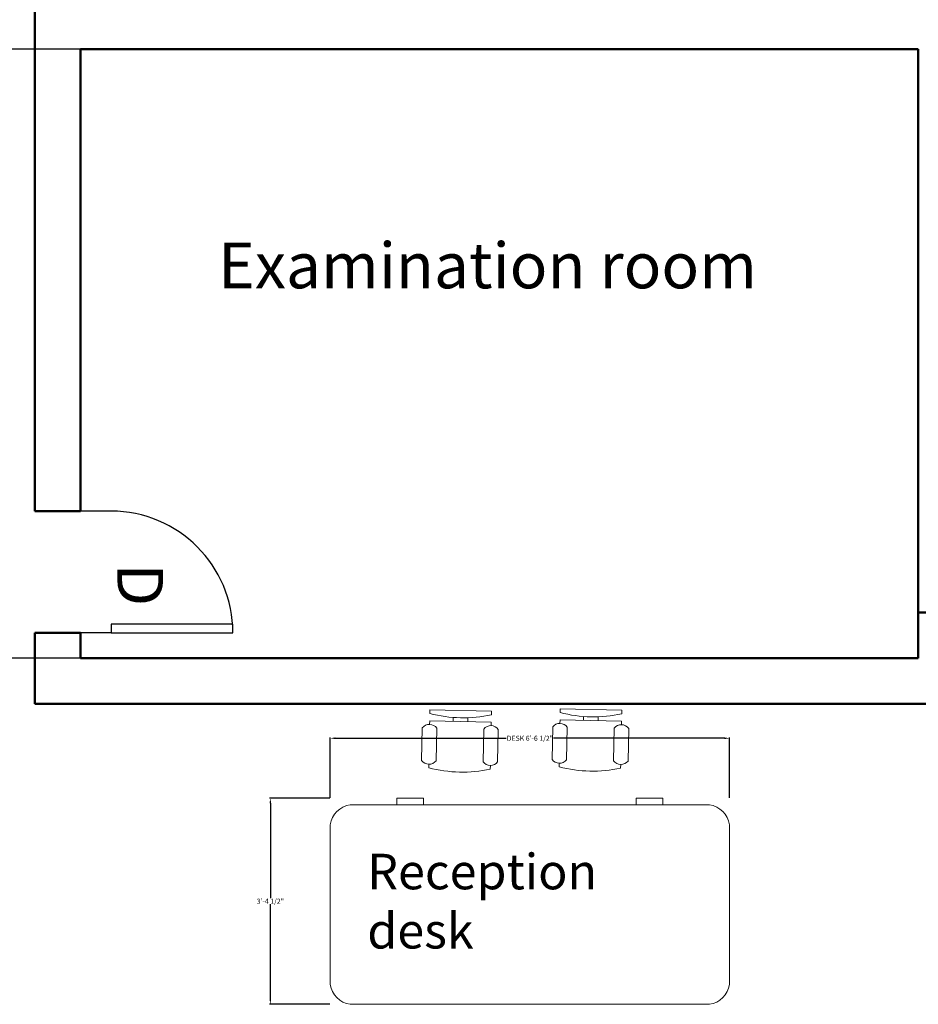
# Model space of a CAD drawing. Units: inches. Extents: x -364 to 705, y -52 to 1250.
# Tile 15 of 34: x 182 to 359, y 454 to 648. Entities that reach past the tile are written whole.
import ezdxf

# ---------------------------------------------------------------- set-up
doc = ezdxf.new("R2010")
doc.units = ezdxf.units.IN
doc.header["$MEASUREMENT"] = 0
for name, color, linetype, lineweight in [('A-ANNO-DIMS', 4, 'Continuous', 18), ('A-ANNO-IDEN', 1, 'Continuous', 18), ('A-ANNO-TEXT', 3, 'Continuous', 18), ('A-AREA-IDEN', 3, 'Continuous', 18), ('A-DOOR', 1, 'Continuous', 25), ('A-FURN', 8, 'Continuous', 18), ('A-WALL', 41, 'Continuous', 50)]:
    doc.layers.add(name, color=color, linetype=linetype, lineweight=lineweight)
doc.styles.get("Standard").update_dxf_attribs({"font": 'arial.ttf'})
doc.dimstyles.get("Standard").update_dxf_attribs({"dimtxt": 1, "dimasz": 1, "dimexe": 0.18, "dimexo": 0.0625, "dimgap": 0.09, "dimtad": 0, "dimtih": 1, "dimtoh": 1, "dimdec": 0, "dimzin": 0, "dimdsep": 46, "dimlunit": 3, "dimtxsty": 'Standard', "dimcen": 0.09, "dimadec": 0, "dimazin": 0, "dimtfac": 1, "dimtdec": 0, "dimtofl": 0, "dimtmove": 0, "dimatfit": 3, "dimfxl": 1, "dimtolj": 1, "dimtzin": 0, "dimarcsym": 0})

# ---------------------------------------------------------------- blocks, each defined once
blk = doc.blocks.new('*U14')
for p, q in [((0, 0), (0, -6)), ((-24, 0), (-24, -6))]:
    blk.add_line(p, q)
blk.add_lwpolyline([(0, 0), (0, 24), (-1.75, 24), (-1.75, 0)], close=True)
blk.add_arc((0, 0), 24, 90, 180)
blk = doc.blocks.new('Chair - Desk')
for p, q in [((-8.5, 0), (-8.5, -1)), ((-8.5, 0), (8.5, 0)), ((8.5, 0), (8.5, -1)), ((-2, -3), (-2, -1.9355)), ((2, -1.9576), (2, -3)), ((-10.5, -5), (-10.5, -14)), ((-8.5, -3), (-8.5, -4)), ((-8.5, -3), (8.5, -3)), ((-6.5, -14), (-6.5, -5)), ((6.5, -5), (6.5, -14)), ((8.5, -3), (8.5, -4)), ((10.5, -14), (10.5, -5)), ((-8.5, -15), (-8.5, -16)), ((8.5, -15), (8.5, -16))]:
    blk.add_line(p, q)
for centre, radius, start, end in [((0, 34.625), 36.625, 256.5803, 283.4197), ((-8.5, -6.5), 2.5, 36.8699, 143.1301), ((8.5, -6.5), 2.5, 36.8699, 143.1301), ((-8.5, -12.5), 2.5, 216.8699, 323.1301), ((0, 19.625), 36.625, 256.5803, 283.4197), ((8.5, -12.5), 2.5, 216.8699, 323.1301)]:
    blk.add_arc(centre, radius, start, end)
blk = doc.blocks.new('Desk - 30 x 60 in.')
for p, q in [((-26.999995, 0), (26.999995, 0)), ((-29.999995, -27), (-29.999995, -3)), ((29.999995, -3), (29.999995, -27)), ((26.999995, -30), (-26.999995, -30)), ((-20.000005, -30), (-20.000005, -31)), ((-20.000005, -31), (-16.000005, -31)), ((-16.000005, -31), (-16.000005, -30)), ((15.999995, -31), (15.999995, -30)), ((19.999995, -31), (15.999995, -31)), ((19.999995, -30), (19.999995, -31))]:
    blk.add_line(p, q)
for centre, start, end in [((-26.499995, -3.5), 98.1301, 171.8699), ((26.499995, -3.5), 8.130102, 81.8699), ((-26.499995, -26.5), 188.1301, 261.8699), ((26.499995, -26.5), 278.1301, 351.8699)]:
    blk.add_arc(centre, 3.535534, start, end)
blk = doc.blocks.new('*D50')
at = {"layer": 'A-ANNO-DIMS', "color": 0, "lineweight": -2, "transparency": 16777216}
for p, q in [((242.75, 494.62), (242.75, 506.53)), ((321.38, 494.62), (321.38, 506.53)), ((243.75, 506.35), (277.41, 506.35)), ((320.38, 506.35), (286.72, 506.35))]:
    blk.add_line(p, q, dxfattribs=at)
at = {"layer": 'A-ANNO-DIMS', "color": 0, "transparency": 16777216}
for points in [[(243.75, 506.52), (243.75, 506.19), (242.75, 506.35)], [(320.38, 506.52), (320.38, 506.19), (321.38, 506.35)]]:
    blk.add_solid(points, dxfattribs=at)
at = {"layer": 'Defpoints', "color": 0, "transparency": 16777216}
for p in [(242.75, 506.35), (242.75, 494.56), (321.38, 494.56)]:
    blk.add_point(p, dxfattribs=at)
at = {"layer": 'A-ANNO-DIMS', "color": 0, "transparency": 16777216, "insert": (282.07, 506.35), "char_height": 1, "attachment_point": 5}
blk.add_mtext('\\A1;DESK 6\'-6 1/2"', dxfattribs=at)
blk = doc.blocks.new('*D51')
at = {"layer": 'A-ANNO-DIMS', "color": 0, "lineweight": -2, "transparency": 16777216}
for p, q in [((242.69, 494.56), (230.77, 494.56)), ((230.95, 493.56), (230.95, 474.85)), ((230.95, 454.93), (230.95, 473.64)), ((242.69, 453.93), (230.77, 453.93))]:
    blk.add_line(p, q, dxfattribs=at)
at = {"layer": 'A-ANNO-DIMS', "color": 0, "transparency": 16777216}
for points in [[(230.79, 493.56), (231.12, 493.56), (230.95, 494.56)], [(230.79, 454.93), (231.12, 454.93), (230.95, 453.93)]]:
    blk.add_solid(points, dxfattribs=at)
at = {"layer": 'Defpoints', "color": 0, "transparency": 16777216}
for p in [(242.75, 494.56), (230.95, 453.93), (242.75, 453.93)]:
    blk.add_point(p, dxfattribs=at)
at = {"layer": 'A-ANNO-DIMS', "color": 0, "transparency": 16777216, "insert": (230.95, 474.24), "char_height": 1, "attachment_point": 5}
blk.add_mtext('\\A1;3\'-4 1/2"', dxfattribs=at)
blk = doc.blocks.new('*D98')
at = {"layer": 'A-ANNO-DIMS', "color": 0, "lineweight": -2, "transparency": 16777216}
for p, q in [((358.52, 642.11), (-126.85, 642.11)), ((-126.67, 641.11), (-126.67, 582.72)), ((-126.67, 523.11), (-126.67, 581.51)), ((358.52, 522.11), (-126.85, 522.11))]:
    blk.add_line(p, q, dxfattribs=at)
at = {"layer": 'A-ANNO-DIMS', "color": 0, "transparency": 16777216}
for points in [[(-126.84, 641.11), (-126.5, 641.11), (-126.67, 642.11)], [(-126.84, 523.11), (-126.5, 523.11), (-126.67, 522.11)]]:
    blk.add_solid(points, dxfattribs=at)
at = {"layer": 'Defpoints', "color": 0, "transparency": 16777216}
for p in [(-126.67, 642.11), (358.58, 642.11), (358.58, 522.11)]:
    blk.add_point(p, dxfattribs=at)
at = {"layer": 'A-ANNO-DIMS', "color": 0, "transparency": 16777216, "insert": (-126.67, 582.11), "char_height": 1, "attachment_point": 5}
blk.add_mtext('\\A1;10\'-0"', dxfattribs=at)

msp = doc.modelspace()

# ---------------------------------------------------------------- linework, layer by layer
at = {"layer": 'A-WALL'}
for p, q in [((184.58, 551.11), (184.58, 656.11)), ((358.58, 642.11), (193.58, 642.11)), ((193.58, 551.11), (193.58, 642.11)), ((358.58, 522.11), (358.58, 642.11)), ((193.58, 551.11), (184.58, 551.11)), ((373.58, 531.11), (358.58, 531.11)), ((184.58, 513.11), (184.58, 527.11)), ((193.58, 527.11), (184.58, 527.11)), ((193.58, 522.11), (193.58, 527.11)), ((358.58, 522.11), (193.58, 522.11)), ((367.58, 513.11), (184.58, 513.11))]:
    msp.add_line(p, q, dxfattribs=at)

# ---------------------------------------------------------------- block references
at = {"layer": 'A-DOOR', "rotation": 270}
msp.add_blockref('*U14', (199.58, 527.11), dxfattribs=at)
at = {"layer": 'A-FURN'}
for name, p, xscale, yscale, zscale, rotation in [('Chair - Desk', (268.44, 511.81), 0.7131197330740188, 0.7131197330740188, 0.7131197330740188, 358.8399543093714), ('Chair - Desk', (294.12, 512), 0.7131197330740188, 0.7131197330740188, 0.7131197330740188, 358.8399543093714), ('Desk - 30 x 60 in.', (282.07, 453.93), 1.310568210035493, 1.310568210035493, 1.310568210035493, 180)]:
    msp.add_blockref(name, p, dxfattribs=dict(at, xscale=xscale, yscale=yscale, zscale=zscale, rotation=rotation))

# ---------------------------------------------------------------- texts
at = {"layer": 'A-ANNO-IDEN', "insert": (209.82, 540.82), "char_height": 9, "attachment_point": 1, "rotation": 270}
msp.add_mtext_dynamic_manual_height_columns('D', width=16.916, gutter_width=1, heights=[0], dxfattribs=at)
at = {"layer": 'A-ANNO-TEXT', "insert": (250.04, 483.59), "char_height": 7, "attachment_point": 1}
msp.add_mtext_dynamic_manual_height_columns('Reception desk', width=47.5468, gutter_width=1, heights=[0], dxfattribs=at)
at = {"layer": 'A-AREA-IDEN', "insert": (220.68, 604.01), "char_height": 9, "attachment_point": 1}
msp.add_mtext_dynamic_manual_height_columns('Examination room', width=124.8937, gutter_width=1, heights=[11.38], dxfattribs=at)

# ---------------------------------------------------------------- dimensions: what is measured, and where the dimension line sits
at = {"layer": 'A-ANNO-DIMS'}
for base, p1, p2, angle, picture, middle in [((-126.67, 642.11), (358.58, 522.11), (358.58, 642.11), 90, '*D98', (-126.67, 582.11)), ((230.95, 453.93), (242.75, 494.56), (242.75, 453.93), 270, '*D51', (230.95, 474.24))]:
    dim = msp.add_linear_dim(base=base, p1=p1, p2=p2, angle=angle, dimstyle='Standard', override={"dimdec": 1, "dimlfac": 1, "dimrnd": 0, "dimzin": 1, "dimdsep": 46, "dimlunit": 4, "dimfrac": 2}, dxfattribs=at)
    dim.commit()
    dim.dimension.update_dxf_attribs({"geometry": picture, "text_midpoint": middle})
dim = msp.add_linear_dim(base=(242.75, 506.35), p1=(321.38, 494.56), p2=(242.75, 494.56), angle=180, text='DESK <>', dimstyle='Standard', override={"dimdec": 1, "dimlfac": 1, "dimrnd": 0, "dimzin": 1, "dimdsep": 46, "dimlunit": 4, "dimfrac": 2}, dxfattribs=at)
dim.commit()
dim.dimension.update_dxf_attribs({"geometry": '*D50', "text_midpoint": (282.07, 506.35)})

doc.saveas('drawing.dxf')
